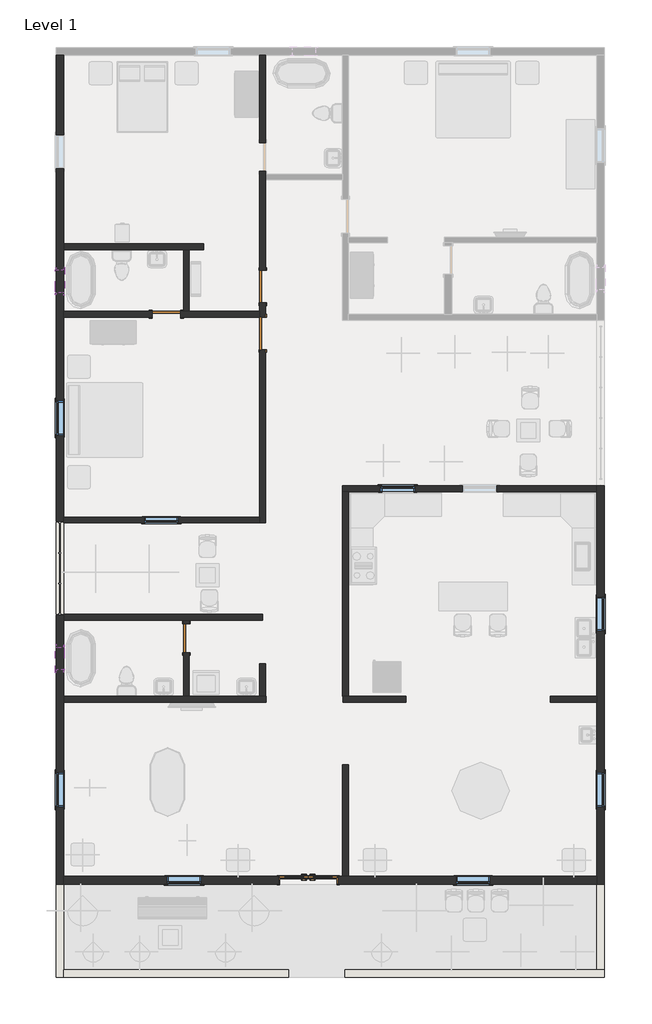
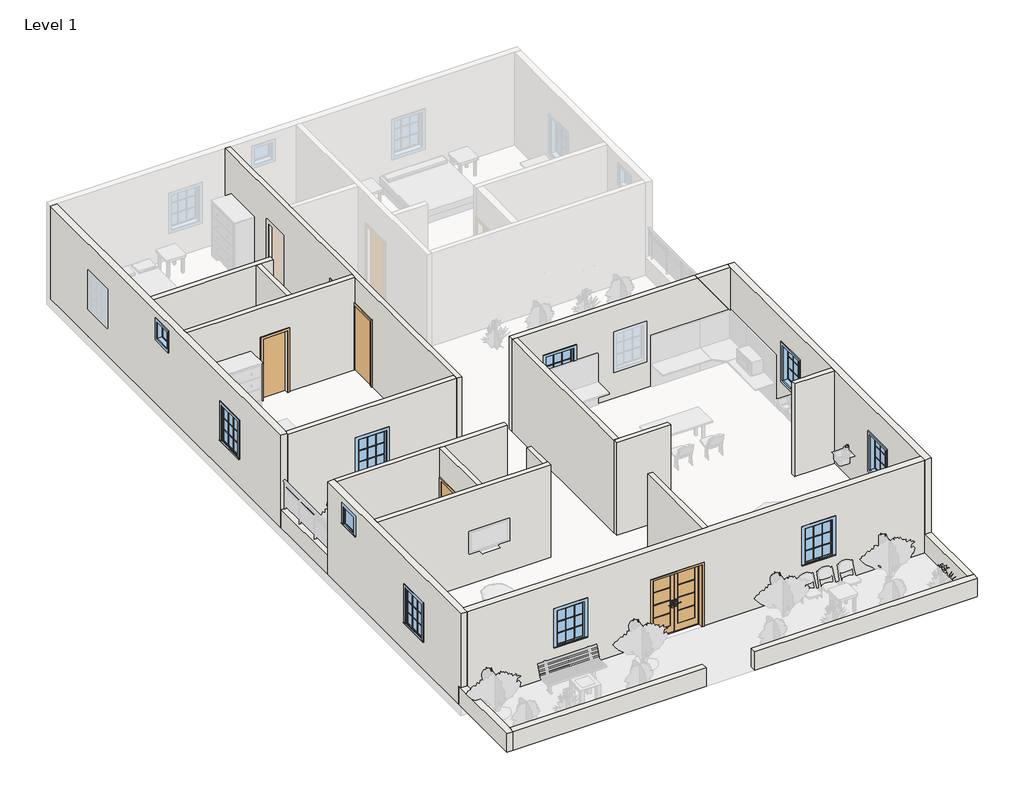
# One storey, part 1 of 3: 23 walls, 10 windows, 5 doors.
"""IFC4 building model written with IfcOpenShell, lengths in millimetres."""

from ifc_helpers import new_model, si_unit, frame, origin, origin_with_axes, place, context, project, spatial, polyline, outline, extrude, faceted_brep, transform, mapped, element, save
from components import door_b03bd389, door_059fdd7e, door_99d96fc5, door_b6e9fca3, window_29c06734, window_5c190c7e, window_e41d21a6

model = new_model("IFC4")

# Units and contexts
model_context = context("Model", 3, world=origin())
ifc_project = project(units=[si_unit("LENGTHUNIT", "METRE", prefix="MILLI")], contexts=[model_context])

# Site, building, storey
site = spatial("IfcSite", under=ifc_project)
building = spatial("IfcBuilding", under=site)
storey = spatial("IfcBuildingStorey", under=building, Name="Level 1", Elevation=0.0)

# Doors
placement = place(None, origin())
door_shape = door_b03bd389(model_context)
element("IfcDoor", 1, ObjectType="Door-Exterior-Double-Full Glass-Wood_Clad : 60\" x 80\"", at=placement, inside=storey, context=model_context, shape_type="MappedRepresentation", body=[
    mapped(door_shape, transform((-8336.7446525, -9537.1247829, 0.0), x_axis=(1.0, 0.0, 0.0), y_axis=(0.0, 1.0, 0.0), z_axis=(0.0, 0.0, 1.0))),
])
door_2_shape = door_059fdd7e(model_context)
element("IfcDoor", 2, ObjectType="Single-Flush : 30\" x 80\"", at=placement, inside=storey, context=model_context, shape_type="MappedRepresentation", body=[
    mapped(door_2_shape, transform((-12121.3446525, 5547.3002171, 0.0), x_axis=(1.0, 0.0, 0.0), y_axis=(0.0, 1.0, 0.0), z_axis=(0.0, 0.0, 1.0))),
])
element("IfcDoor", 3, ObjectType="Single-Flush : 30\" x 80\"", at=placement, inside=storey, context=model_context, shape_type="MappedRepresentation", body=[
    mapped(door_2_shape, transform((-11587.9446525, -3088.6997829, 0.0), x_axis=(0.0, 1.0, 0.0), y_axis=(-1.0, 0.0, 0.0), z_axis=(0.0, 0.0, 1.0))),
])
door_3_shape = door_99d96fc5(model_context)
element("IfcDoor", 4, ObjectType="Single-Flush : 34\" x 84\"", at=placement, inside=storey, context=model_context, shape_type="MappedRepresentation", body=[
    mapped(door_3_shape, transform((-9555.9446525, 6283.9002171, 0.0), x_axis=(0.0, -1.0, 0.0), y_axis=(1.0, 0.0, 0.0), z_axis=(0.0, 0.0, 1.0))),
])
door_4_shape = door_b6e9fca3(model_context)
element("IfcDoor", 5, ObjectType="Single-Flush : 34\" x 84\"", at=placement, inside=storey, context=model_context, shape_type="MappedRepresentation", body=[
    mapped(door_4_shape, transform((-9555.9446525, 5039.3002171, 0.0), x_axis=(0.0, 1.0, 0.0), y_axis=(-1.0, 0.0, 0.0), z_axis=(0.0, 0.0, 1.0))),
])

# Walls
element("IfcWall", 6, ObjectType="Generic - 2'", at=placement, inside=storey, context=model_context, shape_type="Brep", body=[
    faceted_brep([(-14864.5446525, -12131.0997829, 0.0), (-14864.5446525, -11927.8997829, 0.0), (-14864.5446525, -9641.8997829, 0.0), (-14864.5446525, -9540.2997829, 0.0), (-14864.5446525, -9540.2997829, 609.6), (-14864.5446525, -11927.8997829, 609.6), (-14864.5446525, -12131.0997829, 609.6), (-15067.7446525, -12131.0997829, 0.0), (-15067.7446525, -12131.0997829, 609.6), (-15067.7446525, -9540.2997829, 609.6), (-15067.7446525, -9540.2997829, 0.0)], [[[0, 1, 2, 3, 4, 5, 6]], [[7, 8, 9, 10]], [[3, 2, 1, 0, 7, 10]], [[4, 3, 10, 9]], [[6, 5, 4, 9, 8]], [[0, 6, 8, 7]]]),
])
element("IfcWall", 7, ObjectType="Generic - 2'", at=placement, inside=storey, context=model_context, shape_type="SweptSolid", body=[
    extrude(outline(polyline([(-14864.5446525, 10.1002171), (-14864.5446525, -2453.6997829), (-15067.7446525, -2453.6997829), (-15067.7446525, 10.1002171), (-14864.5446525, 10.1002171)])), origin_with_axes(), (0.0, 0.0, 1.0), 609.6),
])
element("IfcWall", 8, ObjectType="Generic - 2'", at=placement, inside=storey, context=model_context, shape_type="SweptSolid", body=[
    extrude(outline(polyline([(-8870.1446525, -12131.0997829), (-14864.5446525, -12131.0997829), (-14864.5446525, -11927.8997829), (-8870.1446525, -11927.8997829), (-8870.1446525, -12131.0997829)])), origin_with_axes(), (0.0, 0.0, 1.0), 609.6),
])
element("IfcWall", 9, ObjectType="Generic - 2'", at=placement, inside=storey, context=model_context, shape_type="Brep", body=[
    faceted_brep([(-7358.8446525, -12131.0997829, 0.0), (-437.3446525, -12131.0997829, 0.0), (-437.3446525, -12131.0997829, 609.6), (-7358.8446525, -12131.0997829, 609.6), (-7358.8446525, -11927.8997829, 0.0), (-7358.8446525, -11927.8997829, 609.6), (-640.5446525, -11927.8997829, 609.6), (-437.3446525, -11927.8997829, 609.6), (-437.3446525, -11927.8997829, 0.0), (-640.5446525, -11927.8997829, 0.0)], [[[0, 1, 2, 3]], [[4, 5, 6, 7, 8, 9]], [[1, 0, 4, 9, 8]], [[3, 2, 7, 6, 5]], [[0, 3, 5, 4]], [[2, 1, 8, 7]]]),
])
element("IfcWall", 10, ObjectType="Generic - 2'", at=placement, inside=storey, context=model_context, shape_type="Brep", body=[
    faceted_brep([(-640.5446525, -9540.2997829, 0.0), (-640.5446525, -9641.8997829, 0.0), (-640.5446525, -11927.8997829, 0.0), (-640.5446525, -11927.8997829, 609.6), (-640.5446525, -9540.2997829, 609.6), (-437.3446525, -9540.2997829, 0.0), (-437.3446525, -9540.2997829, 609.6), (-437.3446525, -11927.8997829, 609.6), (-437.3446525, -11927.8997829, 0.0)], [[[0, 1, 2, 3, 4]], [[5, 6, 7, 8]], [[2, 1, 0, 5, 8]], [[4, 3, 7, 6]], [[0, 4, 6, 5]], [[3, 2, 8, 7]]]),
])
element("IfcWall", 11, ObjectType="Generic - 8\"", at=placement, inside=storey, context=model_context, shape_type="Brep", body=[
    faceted_brep([(-14864.5446525, -9641.8997829, 3048.0), (-14864.5446525, -9641.8997829, 609.6), (-14864.5446525, -9641.8997829, 0.0), (-9124.1446525, -9641.8997829, 0.0), (-9124.1446525, -9641.8997829, 2057.4), (-7549.3446525, -9641.8997829, 2057.4), (-7549.3446525, -9641.8997829, 0.0), (-640.5446525, -9641.8997829, 0.0), (-640.5446525, -9641.8997829, 609.6), (-640.5446525, -9641.8997829, 3048.0), (-12108.6446525, -9641.8997829, 2133.6), (-11194.2446525, -9641.8997829, 2133.6), (-11194.2446525, -9641.8997829, 914.4), (-12108.6446525, -9641.8997829, 914.4), (-4399.7446525, -9641.8997829, 2133.6), (-3485.3446525, -9641.8997829, 2133.6), (-3485.3446525, -9641.8997829, 914.4), (-4399.7446525, -9641.8997829, 914.4), (-14864.5446525, -9438.6997829, 0.0), (-14864.5446525, -9438.6997829, 3048.0), (-7422.3446525, -9438.6997829, 3048.0), (-7269.9446525, -9438.6997829, 3048.0), (-640.5446525, -9438.6997829, 3048.0), (-640.5446525, -9438.6997829, 0.0), (-7269.9446525, -9438.6997829, 0.0), (-7422.3446525, -9438.6997829, 0.0), (-7549.3446525, -9438.6997829, 0.0), (-7549.3446525, -9438.6997829, 2057.4), (-9124.1446525, -9438.6997829, 2057.4), (-9124.1446525, -9438.6997829, 0.0), (-12108.6446525, -9438.6997829, 2133.6), (-12108.6446525, -9438.6997829, 914.4), (-11194.2446525, -9438.6997829, 914.4), (-11194.2446525, -9438.6997829, 2133.6), (-4399.7446525, -9438.6997829, 2133.6), (-4399.7446525, -9438.6997829, 914.4), (-3485.3446525, -9438.6997829, 914.4), (-3485.3446525, -9438.6997829, 2133.6), (-640.5446525, -9540.2997829, 0.0), (-14864.5446525, -9540.2997829, 0.0)], [[[0, 1, 2, 3, 4, 5, 6, 7, 8, 9], [10, 11, 12, 13], [14, 15, 16, 17]], [[18, 19, 20, 21, 22, 23, 24, 25, 26, 27, 28, 29], [30, 31, 32, 33], [34, 35, 36, 37]], [[23, 38, 7, 6, 26, 25, 24]], [[2, 39, 18, 29, 3]], [[5, 27, 26, 6]], [[27, 5, 4, 28]], [[28, 4, 3, 29]], [[31, 30, 10, 13]], [[32, 31, 13, 12]], [[33, 32, 12, 11]], [[30, 33, 11, 10]], [[35, 34, 14, 17]], [[36, 35, 17, 16]], [[37, 36, 16, 15]], [[34, 37, 15, 14]], [[18, 39, 2, 1, 0, 19]], [[7, 38, 23, 22, 9, 8]], [[0, 9, 22, 21, 20, 19]]]),
])
element("IfcWall", 12, ObjectType="Generic - 8\"", at=placement, inside=storey, context=model_context, shape_type="Brep", body=[
    faceted_brep([(-14864.5446525, 35.5002171, 0.0), (-14864.5446525, 137.1002171, 0.0), (-14864.5446525, 5471.1002171, 0.0), (-14864.5446525, 5623.5002171, 0.0), (-14864.5446525, 7274.5002171, 0.0), (-14864.5446525, 7426.9002171, 0.0), (-14864.5446525, 12456.1002171, 0.0), (-14864.5446525, 12456.1002171, 3048.0), (-14864.5446525, 7426.9002171, 3048.0), (-14864.5446525, 7274.5002171, 3048.0), (-14864.5446525, 5623.5002171, 3048.0), (-14864.5446525, 5471.1002171, 3048.0), (-14864.5446525, 137.1002171, 3048.0), (-14864.5446525, 35.5002171, 3048.0), (-14864.5446525, 10335.2002171, 2133.6), (-14864.5446525, 10335.2002171, 914.4), (-14864.5446525, 9420.8002171, 914.4), (-14864.5446525, 9420.8002171, 2133.6), (-14864.5446525, 3235.9002171, 2133.6), (-14864.5446525, 3235.9002171, 914.4), (-14864.5446525, 2321.5002171, 914.4), (-14864.5446525, 2321.5002171, 2133.6), (-14864.5446525, 6118.8002171, 2768.6), (-14864.5446525, 6728.4002171, 2768.6), (-14864.5446525, 6728.4002171, 2159.0), (-14864.5446525, 6118.8002171, 2159.0), (-15067.7446525, 35.5002171, 0.0), (-15067.7446525, 35.5002171, 3048.0), (-15067.7446525, 12456.1002171, 3048.0), (-15067.7446525, 12456.1002171, 0.0), (-15067.7446525, 10335.2002171, 2133.6), (-15067.7446525, 9420.8002171, 2133.6), (-15067.7446525, 9420.8002171, 914.4), (-15067.7446525, 10335.2002171, 914.4), (-15067.7446525, 3235.9002171, 2133.6), (-15067.7446525, 2321.5002171, 2133.6), (-15067.7446525, 2321.5002171, 914.4), (-15067.7446525, 3235.9002171, 914.4), (-15067.7446525, 6118.8002171, 2768.6), (-15067.7446525, 6118.8002171, 2159.0), (-15067.7446525, 6728.4002171, 2159.0), (-15067.7446525, 6728.4002171, 2768.6)], [[[0, 1, 2, 3, 4, 5, 6, 7, 8, 9, 10, 11, 12, 13], [14, 15, 16, 17], [18, 19, 20, 21], [22, 23, 24, 25]], [[26, 27, 28, 29], [30, 31, 32, 33], [34, 35, 36, 37], [38, 39, 40, 41]], [[6, 5, 4, 3, 2, 1, 0, 26, 29]], [[0, 13, 27, 26]], [[7, 6, 29, 28]], [[15, 14, 30, 33]], [[16, 15, 33, 32]], [[17, 16, 32, 31]], [[14, 17, 31, 30]], [[19, 18, 34, 37]], [[20, 19, 37, 36]], [[21, 20, 36, 35]], [[18, 21, 35, 34]], [[39, 38, 22, 25]], [[40, 39, 25, 24]], [[41, 40, 24, 23]], [[38, 41, 23, 22]], [[13, 12, 11, 10, 9, 8, 7, 28, 27]]]),
])
element("IfcWall", 13, ObjectType="Generic - 8\"", at=placement, inside=storey, context=model_context, shape_type="Brep", body=[
    faceted_brep([(-640.5446525, 899.1002171, 0.0), (-640.5446525, 822.9002171, 0.0), (-640.5446525, -4638.0997829, 0.0), (-640.5446525, -4790.4997829, 0.0), (-640.5446525, -9438.6997829, 0.0), (-640.5446525, -9540.2997829, 0.0), (-640.5446525, -9540.2997829, 609.6), (-640.5446525, -9641.8997829, 609.6), (-640.5446525, -9641.8997829, 3048.0), (-640.5446525, -9438.6997829, 3048.0), (-640.5446525, -4790.4997829, 3048.0), (-640.5446525, -4638.0997829, 3048.0), (-640.5446525, 822.9002171, 3048.0), (-640.5446525, 975.3002171, 3048.0), (-640.5446525, 975.3002171, 609.6), (-640.5446525, 899.1002171, 609.6), (-640.5446525, -7584.4997829, 2133.6), (-640.5446525, -7584.4997829, 914.4), (-640.5446525, -6670.0997829, 914.4), (-640.5446525, -6670.0997829, 2133.6), (-640.5446525, -2898.1997829, 2228.85), (-640.5446525, -2898.1997829, 1009.65), (-640.5446525, -1983.7997829, 1009.65), (-640.5446525, -1983.7997829, 2228.85), (-437.3446525, 899.1002171, 0.0), (-437.3446525, 899.1002171, 609.6), (-437.3446525, 975.3002171, 609.6), (-437.3446525, 975.3002171, 3048.0), (-437.3446525, -9641.8997829, 3048.0), (-437.3446525, -9641.8997829, 609.6), (-437.3446525, -9540.2997829, 609.6), (-437.3446525, -9540.2997829, 0.0), (-437.3446525, -7584.4997829, 2133.6), (-437.3446525, -6670.0997829, 2133.6), (-437.3446525, -6670.0997829, 914.4), (-437.3446525, -7584.4997829, 914.4), (-437.3446525, -2898.1997829, 2228.85), (-437.3446525, -1983.7997829, 2228.85), (-437.3446525, -1983.7997829, 1009.65), (-437.3446525, -2898.1997829, 1009.65)], [[[0, 1, 2, 3, 4, 5, 6, 7, 8, 9, 10, 11, 12, 13, 14, 15], [16, 17, 18, 19], [20, 21, 22, 23]], [[24, 25, 26, 27, 28, 29, 30, 31], [32, 33, 34, 35], [36, 37, 38, 39]], [[5, 4, 3, 2, 1, 0, 24, 31]], [[16, 19, 33, 32]], [[19, 18, 34, 33]], [[18, 17, 35, 34]], [[17, 16, 32, 35]], [[20, 23, 37, 36]], [[23, 22, 38, 37]], [[22, 21, 39, 38]], [[21, 20, 36, 39]], [[0, 15, 25, 24]], [[14, 26, 25, 15]], [[14, 13, 27, 26]], [[6, 5, 31, 30]], [[29, 7, 6, 30]], [[8, 7, 29, 28]], [[13, 12, 11, 10, 9, 8, 28, 27]]]),
])
element("IfcWall", 14, ObjectType="Generic - 8\"", at=placement, inside=storey, context=model_context, shape_type="Brep", body=[
    faceted_brep([(-14864.5446525, -9540.2997829, 0.0), (-14864.5446525, -9438.6997829, 0.0), (-14864.5446525, -4790.4997829, 0.0), (-14864.5446525, -4638.0997829, 0.0), (-14864.5446525, -2606.0997829, 0.0), (-14864.5446525, -2479.0997829, 0.0), (-14864.5446525, -2479.0997829, 3048.0), (-14864.5446525, -2606.0997829, 3048.0), (-14864.5446525, -4638.0997829, 3048.0), (-14864.5446525, -4790.4997829, 3048.0), (-14864.5446525, -9438.6997829, 3048.0), (-14864.5446525, -9641.8997829, 3048.0), (-14864.5446525, -9641.8997829, 609.6), (-14864.5446525, -9540.2997829, 609.6), (-14864.5446525, -6670.0997829, 2133.6), (-14864.5446525, -6670.0997829, 914.4), (-14864.5446525, -7584.4997829, 914.4), (-14864.5446525, -7584.4997829, 2133.6), (-14864.5446525, -3323.6497829, 2768.6), (-14864.5446525, -3323.6497829, 2159.0), (-14864.5446525, -3933.2497829, 2159.0), (-14864.5446525, -3933.2497829, 2768.6), (-15067.7446525, -9540.2997829, 0.0), (-15067.7446525, -9540.2997829, 609.6), (-15067.7446525, -9641.8997829, 609.6), (-15067.7446525, -9641.8997829, 3048.0), (-15067.7446525, -2479.0997829, 3048.0), (-15067.7446525, -2479.0997829, 0.0), (-15067.7446525, -6670.0997829, 2133.6), (-15067.7446525, -7584.4997829, 2133.6), (-15067.7446525, -7584.4997829, 914.4), (-15067.7446525, -6670.0997829, 914.4), (-15067.7446525, -3323.6497829, 2768.6), (-15067.7446525, -3933.2497829, 2768.6), (-15067.7446525, -3933.2497829, 2159.0), (-15067.7446525, -3323.6497829, 2159.0)], [[[0, 1, 2, 3, 4, 5, 6, 7, 8, 9, 10, 11, 12, 13], [14, 15, 16, 17], [18, 19, 20, 21]], [[22, 23, 24, 25, 26, 27], [28, 29, 30, 31], [32, 33, 34, 35]], [[5, 4, 3, 2, 1, 0, 22, 27]], [[6, 5, 27, 26]], [[14, 17, 29, 28]], [[17, 16, 30, 29]], [[16, 15, 31, 30]], [[15, 14, 28, 31]], [[18, 21, 33, 32]], [[21, 20, 34, 33]], [[20, 19, 35, 34]], [[19, 18, 32, 35]], [[0, 13, 23, 22]], [[12, 24, 23, 13]], [[12, 11, 25, 24]], [[11, 10, 9, 8, 7, 6, 26, 25]]]),
])
element("IfcWall", 15, ObjectType="INNER 6\"", at=placement, inside=storey, context=model_context, shape_type="SweptSolid", body=[
    extrude(outline(polyline([(-1885.1446525, -4638.0997829), (-640.5446525, -4638.0997829), (-640.5446525, -4790.4997829), (-1885.1446525, -4790.4997829), (-1885.1446525, -4638.0997829)])), origin_with_axes(), (0.0, 0.0, 1.0), 3048.0),
])
element("IfcWall", 16, ObjectType="INNER 6\"", at=placement, inside=storey, context=model_context, shape_type="Brep", body=[
    faceted_brep([(-9632.1446525, 5852.1002171, 0.0), (-9632.1446525, 5623.5002171, 0.0), (-9632.1446525, 5471.1002171, 0.0), (-9632.1446525, 5471.1002171, 2133.6), (-9632.1446525, 4607.5002171, 2133.6), (-9632.1446525, 4607.5002171, 0.0), (-9632.1446525, 137.1002171, 0.0), (-9632.1446525, -15.2997829, 0.0), (-9632.1446525, -15.2997829, 3048.0), (-9632.1446525, 137.1002171, 3048.0), (-9632.1446525, 5471.1002171, 3048.0), (-9632.1446525, 5623.5002171, 3048.0), (-9632.1446525, 12456.1002171, 3048.0), (-9632.1446525, 12456.1002171, 0.0), (-9632.1446525, 10119.3002171, 0.0), (-9632.1446525, 10119.3002171, 2032.0), (-9632.1446525, 9357.3002171, 2032.0), (-9632.1446525, 9357.3002171, 0.0), (-9632.1446525, 6715.7002171, 0.0), (-9632.1446525, 6715.7002171, 2133.6), (-9632.1446525, 5852.1002171, 2133.6), (-9479.7446525, 5471.1002171, 2133.6), (-9479.7446525, 5471.1002171, 0.0), (-9479.7446525, 5852.1002171, 0.0), (-9479.7446525, 5852.1002171, 2133.6), (-9479.7446525, 6715.7002171, 2133.6), (-9479.7446525, 6715.7002171, 0.0), (-9479.7446525, 9128.7002171, 0.0), (-9479.7446525, 9281.1002171, 0.0), (-9479.7446525, 9357.3002171, 0.0), (-9479.7446525, 9357.3002171, 2032.0), (-9479.7446525, 10119.3002171, 2032.0), (-9479.7446525, 10119.3002171, 0.0), (-9479.7446525, 12456.1002171, 0.0), (-9479.7446525, 12456.1002171, 3048.0), (-9479.7446525, 9281.1002171, 3048.0), (-9479.7446525, 9128.7002171, 3048.0), (-9479.7446525, -15.2997829, 3048.0), (-9479.7446525, -15.2997829, 0.0), (-9479.7446525, 4607.5002171, 0.0), (-9479.7446525, 4607.5002171, 2133.6)], [[[0, 1, 2, 3, 4, 5, 6, 7, 8, 9, 10, 11, 12, 13, 14, 15, 16, 17, 18, 19, 20]], [[21, 22, 23, 24, 25, 26, 27, 28, 29, 30, 31, 32, 33, 34, 35, 36, 37, 38, 39, 40]], [[14, 13, 33, 32]], [[18, 17, 29, 28, 27, 26]], [[39, 38, 7, 6, 5]], [[23, 22, 2, 1, 0]], [[13, 12, 34, 33]], [[8, 7, 38, 37]], [[30, 29, 17, 16]], [[31, 30, 16, 15]], [[32, 31, 15, 14]], [[24, 23, 0, 20]], [[25, 24, 20, 19]], [[26, 25, 19, 18]], [[3, 2, 22, 21]], [[4, 3, 21, 40]], [[5, 4, 40, 39]], [[12, 11, 10, 9, 8, 37, 36, 35, 34]]]),
])
element("IfcWall", 17, ObjectType="INNER 6\"", at=placement, inside=storey, context=model_context, shape_type="Brep", body=[
    faceted_brep([(-9632.1446525, 5623.5002171, 0.0), (-11511.7446525, 5623.5002171, 0.0), (-11664.1446525, 5623.5002171, 0.0), (-11740.3446525, 5623.5002171, 0.0), (-11740.3446525, 5623.5002171, 2032.0), (-12502.3446525, 5623.5002171, 2032.0), (-12502.3446525, 5623.5002171, 0.0), (-14864.5446525, 5623.5002171, 0.0), (-14864.5446525, 5623.5002171, 3048.0), (-11664.1446525, 5623.5002171, 3048.0), (-11511.7446525, 5623.5002171, 3048.0), (-9632.1446525, 5623.5002171, 3048.0), (-11740.3446525, 5471.1002171, 2032.0), (-11740.3446525, 5471.1002171, 0.0), (-9632.1446525, 5471.1002171, 0.0), (-9632.1446525, 5471.1002171, 2133.6), (-9632.1446525, 5471.1002171, 3048.0), (-14864.5446525, 5471.1002171, 3048.0), (-14864.5446525, 5471.1002171, 0.0), (-12502.3446525, 5471.1002171, 0.0), (-12502.3446525, 5471.1002171, 2032.0)], [[[0, 1, 2, 3, 4, 5, 6, 7, 8, 9, 10, 11]], [[12, 13, 14, 15, 16, 17, 18, 19, 20]], [[19, 18, 7, 6]], [[14, 13, 3, 2, 1, 0]], [[0, 11, 16, 15, 14]], [[8, 7, 18, 17]], [[4, 3, 13, 12]], [[5, 4, 12, 20]], [[6, 5, 20, 19]], [[11, 10, 9, 8, 17, 16]]]),
])
element("IfcWall", 18, ObjectType="INNER 6\"", at=placement, inside=storey, context=model_context, shape_type="Brep", body=[
    faceted_brep([(-14864.5446525, 7274.5002171, 0.0), (-11664.1446525, 7274.5002171, 0.0), (-11511.7446525, 7274.5002171, 0.0), (-11130.7446525, 7274.5002171, 0.0), (-11130.7446525, 7274.5002171, 3048.0), (-11511.7446525, 7274.5002171, 3048.0), (-11664.1446525, 7274.5002171, 3048.0), (-14864.5446525, 7274.5002171, 3048.0), (-14864.5446525, 7426.9002171, 0.0), (-14864.5446525, 7426.9002171, 3048.0), (-11130.7446525, 7426.9002171, 3048.0), (-11130.7446525, 7426.9002171, 0.0)], [[[0, 1, 2, 3, 4, 5, 6, 7]], [[8, 9, 10, 11]], [[3, 2, 1, 0, 8, 11]], [[4, 3, 11, 10]], [[0, 7, 9, 8]], [[7, 6, 5, 4, 10, 9]]]),
])
element("IfcWall", 19, ObjectType="INNER 6\"", at=placement, inside=storey, context=model_context, shape_type="SweptSolid", body=[
    extrude(outline(polyline([(-11664.1446525, 5623.5002171), (-11664.1446525, 7274.5002171), (-11511.7446525, 7274.5002171), (-11511.7446525, 5623.5002171), (-11664.1446525, 5623.5002171)])), origin_with_axes(), (0.0, 0.0, 1.0), 3048.0),
])
element("IfcWall", 20, ObjectType="INNER 6\"", at=placement, inside=storey, context=model_context, shape_type="Brep", body=[
    faceted_brep([(-9632.1446525, 137.1002171, 0.0), (-14864.5446525, 137.1002171, 0.0), (-14864.5446525, 137.1002171, 3048.0), (-9632.1446525, 137.1002171, 3048.0), (-12718.2446525, 137.1002171, 2133.6), (-12718.2446525, 137.1002171, 914.4), (-11803.8446525, 137.1002171, 914.4), (-11803.8446525, 137.1002171, 2133.6), (-9632.1446525, -15.2997829, 0.0), (-9632.1446525, -15.2997829, 3048.0), (-14864.5446525, -15.2997829, 3048.0), (-14864.5446525, -15.2997829, 0.0), (-12718.2446525, -15.2997829, 2133.6), (-11803.8446525, -15.2997829, 2133.6), (-11803.8446525, -15.2997829, 914.4), (-12718.2446525, -15.2997829, 914.4), (-14864.5446525, 35.5002171, 0.0), (-14864.5446525, 35.5002171, 3048.0)], [[[0, 1, 2, 3], [4, 5, 6, 7]], [[8, 9, 10, 11], [12, 13, 14, 15]], [[1, 0, 8, 11, 16]], [[0, 3, 9, 8]], [[2, 1, 16, 11, 10, 17]], [[5, 4, 12, 15]], [[6, 5, 15, 14]], [[7, 6, 14, 13]], [[4, 7, 13, 12]], [[3, 2, 17, 10, 9]]]),
])
element("IfcWall", 21, ObjectType="INNER 6\"", at=placement, inside=storey, context=model_context, shape_type="Brep", body=[
    faceted_brep([(-9555.9446525, -2453.6997829, 0.0), (-14864.5446525, -2453.6997829, 0.0), (-14864.5446525, -2453.6997829, 3048.0), (-9555.9446525, -2453.6997829, 3048.0), (-9555.9446525, -2606.0997829, 0.0), (-9555.9446525, -2606.0997829, 3048.0), (-11511.7446525, -2606.0997829, 3048.0), (-11664.1446525, -2606.0997829, 3048.0), (-14864.5446525, -2606.0997829, 3048.0), (-14864.5446525, -2606.0997829, 0.0), (-11664.1446525, -2606.0997829, 0.0), (-11511.7446525, -2606.0997829, 0.0), (-14864.5446525, -2479.0997829, 0.0), (-14864.5446525, -2479.0997829, 3048.0)], [[[0, 1, 2, 3]], [[4, 5, 6, 7, 8, 9, 10, 11]], [[1, 0, 4, 11, 10, 9, 12]], [[0, 3, 5, 4]], [[2, 1, 12, 9, 8, 13]], [[3, 2, 13, 8, 7, 6, 5]]]),
])
element("IfcWall", 22, ObjectType="INNER 6\"", at=placement, inside=storey, context=model_context, shape_type="SweptSolid", body=[
    extrude(outline(polyline([(-2606.0997829, 0.0), (-2707.6997829, 0.0), (-2707.6997829, 2032.0), (-3469.6997829, 2032.0), (-3469.6997829, 0.0), (-4638.0997829, 0.0), (-4638.0997829, 3048.0), (-2606.0997829, 3048.0), (-2606.0997829, 0.0)])), frame((-11664.1446525, 0.0, 0.0), z_axis=(1.0, 0.0, 0.0), x_axis=(0.0, 1.0, 0.0)), (0.0, 0.0, 1.0), 152.4),
])
element("IfcWall", 23, ObjectType="INNER 6\"", at=placement, inside=storey, context=model_context, shape_type="Brep", body=[
    faceted_brep([(-7422.3446525, 822.9002171, 0.0), (-7269.9446525, 822.9002171, 0.0), (-640.5446525, 822.9002171, 0.0), (-640.5446525, 822.9002171, 3048.0), (-7269.9446525, 822.9002171, 3048.0), (-7422.3446525, 822.9002171, 3048.0), (-3307.5446525, 822.9002171, 2133.6), (-3307.5446525, 822.9002171, 914.4), (-4221.9446525, 822.9002171, 914.4), (-4221.9446525, 822.9002171, 2133.6), (-5491.9446525, 822.9002171, 2133.6), (-5491.9446525, 822.9002171, 914.4), (-6406.3446525, 822.9002171, 914.4), (-6406.3446525, 822.9002171, 2133.6), (-7422.3446525, 975.3002171, 0.0), (-7422.3446525, 975.3002171, 3048.0), (-640.5446525, 975.3002171, 3048.0), (-640.5446525, 975.3002171, 609.6), (-640.5446525, 975.3002171, 0.0), (-3307.5446525, 975.3002171, 2133.6), (-4221.9446525, 975.3002171, 2133.6), (-4221.9446525, 975.3002171, 914.4), (-3307.5446525, 975.3002171, 914.4), (-5491.9446525, 975.3002171, 2133.6), (-6406.3446525, 975.3002171, 2133.6), (-6406.3446525, 975.3002171, 914.4), (-5491.9446525, 975.3002171, 914.4), (-640.5446525, 899.1002171, 0.0)], [[[0, 1, 2, 3, 4, 5], [6, 7, 8, 9], [10, 11, 12, 13]], [[14, 15, 16, 17, 18], [19, 20, 21, 22], [23, 24, 25, 26]], [[2, 1, 0, 14, 18, 27]], [[0, 5, 15, 14]], [[7, 6, 19, 22]], [[8, 7, 22, 21]], [[9, 8, 21, 20]], [[6, 9, 20, 19]], [[11, 10, 23, 26]], [[12, 11, 26, 25]], [[13, 12, 25, 24]], [[10, 13, 24, 23]], [[2, 27, 18, 17, 16, 3]], [[5, 4, 3, 16, 15]]]),
])
element("IfcWall", 24, ObjectType="INNER 6\"", at=placement, inside=storey, context=model_context, shape_type="Brep", body=[
    faceted_brep([(-7422.3446525, 822.9002171, 0.0), (-7422.3446525, -4638.0997829, 0.0), (-7422.3446525, -4638.0997829, 3048.0), (-7422.3446525, 822.9002171, 3048.0), (-7269.9446525, 822.9002171, 0.0), (-7269.9446525, 822.9002171, 3048.0), (-7269.9446525, -4638.0997829, 3048.0), (-7269.9446525, -4638.0997829, 0.0), (-7409.6446525, -4638.0997829, 0.0), (-7409.6446525, -4638.0997829, 3048.0)], [[[0, 1, 2, 3]], [[4, 5, 6, 7]], [[1, 0, 4, 7, 8]], [[0, 3, 5, 4]], [[2, 1, 8, 7, 6, 9]], [[3, 2, 9, 6, 5]]]),
])
element("IfcWall", 25, ObjectType="INNER 6\"", at=placement, inside=storey, context=model_context, shape_type="SweptSolid", body=[
    extrude(outline(polyline([(-7422.3446525, -9438.6997829), (-7422.3446525, -6466.8997829), (-7269.9446525, -6466.8997829), (-7269.9446525, -9438.6997829), (-7422.3446525, -9438.6997829)])), origin_with_axes(), (0.0, 0.0, 1.0), 3048.0),
])
element("IfcWall", 26, ObjectType="INNER 6\"", at=placement, inside=storey, context=model_context, shape_type="SweptSolid", body=[
    extrude(outline(polyline([(-9632.1446525, -4638.0997829), (-9632.1446525, -3774.4997829), (-9479.7446525, -3774.4997829), (-9479.7446525, -4638.0997829), (-9632.1446525, -4638.0997829)])), origin_with_axes(), (0.0, 0.0, 1.0), 3048.0),
])
element("IfcWall", 27, ObjectType="INNER 6\"", at=placement, inside=storey, context=model_context, shape_type="Brep", body=[
    faceted_brep([(-9467.0446525, -4638.0997829, 0.0), (-9479.7446525, -4638.0997829, 0.0), (-9632.1446525, -4638.0997829, 0.0), (-11511.7446525, -4638.0997829, 0.0), (-11664.1446525, -4638.0997829, 0.0), (-14864.5446525, -4638.0997829, 0.0), (-14864.5446525, -4638.0997829, 3048.0), (-11664.1446525, -4638.0997829, 3048.0), (-11511.7446525, -4638.0997829, 3048.0), (-9632.1446525, -4638.0997829, 3048.0), (-9479.7446525, -4638.0997829, 3048.0), (-9467.0446525, -4638.0997829, 3048.0), (-9467.0446525, -4790.4997829, 0.0), (-9467.0446525, -4790.4997829, 3048.0), (-14864.5446525, -4790.4997829, 3048.0), (-14864.5446525, -4790.4997829, 0.0)], [[[0, 1, 2, 3, 4, 5, 6, 7, 8, 9, 10, 11]], [[12, 13, 14, 15]], [[5, 4, 3, 2, 1, 0, 12, 15]], [[0, 11, 13, 12]], [[6, 5, 15, 14]], [[11, 10, 9, 8, 7, 6, 14, 13]]]),
])
element("IfcWall", 28, ObjectType="INNER 6\"", at=placement, inside=storey, context=model_context, shape_type="Brep", body=[
    faceted_brep([(-5733.2446525, -4638.0997829, 0.0), (-7269.9446525, -4638.0997829, 0.0), (-7409.6446525, -4638.0997829, 0.0), (-7409.6446525, -4638.0997829, 3048.0), (-7269.9446525, -4638.0997829, 3048.0), (-5733.2446525, -4638.0997829, 3048.0), (-5733.2446525, -4790.4997829, 0.0), (-5733.2446525, -4790.4997829, 3048.0), (-7409.6446525, -4790.4997829, 3048.0), (-7409.6446525, -4790.4997829, 0.0)], [[[0, 1, 2, 3, 4, 5]], [[6, 7, 8, 9]], [[2, 1, 0, 6, 9]], [[3, 2, 9, 8]], [[0, 5, 7, 6]], [[5, 4, 3, 8, 7]]]),
])

# Windows
window_shape = window_29c06734(model_context)
element("IfcWindow", 29, ObjectType="Casement 3x3 with Trim : 36\" x 48\"", at=placement, inside=storey, context=model_context, shape_type="MappedRepresentation", body=[
    mapped(window_shape, transform((-14966.1446525, 2778.7002171, 0.0), x_axis=(0.0, 1.0, 0.0), y_axis=(-1.0, 0.0, 0.0), z_axis=(0.0, 0.0, 1.0))),
])
element("IfcWindow", 30, ObjectType="Casement 3x3 with Trim : 36\" x 48\"", at=placement, inside=storey, context=model_context, shape_type="MappedRepresentation", body=[
    mapped(window_shape, transform((-14966.1446525, -7127.2997829, 0.0), x_axis=(0.0, 1.0, 0.0), y_axis=(-1.0, 0.0, 0.0), z_axis=(0.0, 0.0, 1.0))),
])
element("IfcWindow", 31, ObjectType="Casement 3x3 with Trim : 36\" x 48\"", at=placement, inside=storey, context=model_context, shape_type="MappedRepresentation", body=[
    mapped(window_shape, transform((-11651.4446525, -9540.2997829, 0.0), x_axis=(-1.0, 0.0, 0.0), y_axis=(0.0, -1.0, 0.0), z_axis=(0.0, 0.0, 1.0))),
])
element("IfcWindow", 32, ObjectType="Casement 3x3 with Trim : 36\" x 48\"", at=placement, inside=storey, context=model_context, shape_type="MappedRepresentation", body=[
    mapped(window_shape, transform((-3942.5446525, -9540.2997829, 0.0), x_axis=(-1.0, 0.0, 0.0), y_axis=(0.0, -1.0, 0.0), z_axis=(0.0, 0.0, 1.0))),
])
element("IfcWindow", 33, ObjectType="Casement 3x3 with Trim : 36\" x 48\"", at=placement, inside=storey, context=model_context, shape_type="MappedRepresentation", body=[
    mapped(window_shape, transform((-538.9446525, -7127.2997829, 0.0), x_axis=(0.0, -1.0, 0.0), y_axis=(1.0, 0.0, 0.0), z_axis=(0.0, 0.0, 1.0))),
])
element("IfcWindow", 34, ObjectType="Casement 3x3 with Trim : 36\" x 48\"", at=placement, inside=storey, context=model_context, shape_type="MappedRepresentation", body=[
    mapped(window_shape, transform((-538.9446525, -2440.9997829, 95.25), x_axis=(0.0, -1.0, 0.0), y_axis=(1.0, 0.0, 0.0), z_axis=(0.0, 0.0, 1.0))),
])
window_2_shape = window_5c190c7e(model_context)
element("IfcWindow", 35, ObjectType="Casement 3x3 with Trim : 36\" x 48\"", at=placement, inside=storey, context=model_context, shape_type="MappedRepresentation", body=[
    mapped(window_2_shape, transform((-12261.0446525, 60.9002171, 0.0), x_axis=(-1.0, 0.0, 0.0), y_axis=(0.0, -1.0, 0.0), z_axis=(0.0, 0.0, 1.0))),
])
element("IfcWindow", 36, ObjectType="Casement 3x3 with Trim : 36\" x 48\"", at=placement, inside=storey, context=model_context, shape_type="MappedRepresentation", body=[
    mapped(window_2_shape, transform((-5949.1446525, 899.1002171, 0.0), x_axis=(1.0, 0.0, 0.0), y_axis=(0.0, 1.0, 0.0), z_axis=(0.0, 0.0, 1.0))),
])
window_3_shape = window_e41d21a6(model_context)
element("IfcWindow", 37, ObjectType="Transom with Trim : 24\" x 24\"", at=placement, inside=storey, context=model_context, shape_type="MappedRepresentation", body=[
    mapped(window_3_shape, transform((-14966.1446525, 6385.5002171, 0.0), x_axis=(0.0, -1.0, 0.0), y_axis=(1.0, 0.0, 0.0), z_axis=(0.0, 0.0, 1.0))),
])
element("IfcWindow", 38, ObjectType="Transom with Trim : 24\" x 24\"", at=placement, inside=storey, context=model_context, shape_type="MappedRepresentation", body=[
    mapped(window_3_shape, transform((-14966.1446525, -3590.3497829, 0.0), x_axis=(0.0, 1.0, 0.0), y_axis=(-1.0, 0.0, 0.0), z_axis=(0.0, 0.0, 1.0))),
])

save(model, "model.ifc")

# Revit data of these elements
# Type "Door-Exterior-Double-Full Glass-Wood_Clad : 60\" x 80\""
#   Type Mark = "8"
#   Assembly Code = "B2030100"
#   Analytic Construction = "French door, wood frame with double glass"
#   Top Rail = 0' - 4 11/16"
#   Threshold Offset [instance default] = 0' - 0 1/2"
#   Thickness = 0' - 1 3/8"
#   Thermal Resistance (R) = 1.9158 (h·ft²·°F)/BTU
#   Swing Angle [instance default] = 90.00°
#   Stiles = 0' - 4 3/4"
#   Rough Width = 5' - 2"
#   Rough Height = 6' - 9"
#   Panel Width = 2' - 6"
#   Door Offset [instance default] = 0' - 0"
#   Height = 6' - 8"
#   Width = 5' - 0"
#   Heat Transfer Coefficient (U) = 0.5220 BTU/(h·ft²·°F)
#   Bottom Rail = 0' - 9 1/8"
#   Exterior Trim [instance default] = yes
#   Threshold [instance default] = yes
#   Show Grill [instance default] = yes
#   Function = 1
#   Trim Material = Cherry
#   Threshold Material = Cherry
#   Panel Material = Cherry
#   Glazing = Glass
#   Frame Material = Cherry
#   Door Handle Material = Aluminum
#   Visual Light Transmittance = 0
#   Solar Heat Gain Coefficient = 0
#   Wall Closure = (empty or 0)
#   Construction Type = (empty or 0)
# Type "Single-Flush : 30\" x 80\""
#   Type Mark = "5"
#   Construction Type Id = "MDOOR"
#   Assembly Code = "C1020"
#   Analytic Construction = "Metal"
#   Thickness = 0' - 2"
#   Heat Transfer Coefficient (U) = 0.651978 BTU/(h·ft²·°F)
#   Height = 6' - 8"
#   Trim Projection Ext = 0' - 1"
#   Trim Projection Int = 0' - 1"
#   Trim Width = 0' - 3"
#   Width = 2' - 6"
#   Define Thermal Properties by = 1
#   Door Material = Door - Panel
#   Frame Material = Door - Frame
#   Visual Light Transmittance = 0
#   Solar Heat Gain Coefficient = 0
#   Function = (empty or 0)
#   Wall Closure = (empty or 0)
# Type "Single-Flush : 34\" x 84\""
#   Type Mark = "2"
#   Construction Type Id = "MDOOR"
#   Assembly Code = "C1020"
#   Analytic Construction = "Metal"
#   Thickness = 0' - 2"
#   Heat Transfer Coefficient (U) = 0.651978 BTU/(h·ft²·°F)
#   Height = 7' - 0"
#   Trim Projection Ext = 0' - 1"
#   Trim Projection Int = 0' - 1"
#   Trim Width = 0' - 3"
#   Width = 2' - 10"
#   Define Thermal Properties by = 1
#   Door Material = Door - Panel
#   Frame Material = Door - Frame
#   Visual Light Transmittance = 0
#   Solar Heat Gain Coefficient = 0
#   Function = (empty or 0)
#   Wall Closure = (empty or 0)
# Type "Generic - 2'"
#   Assembly Code = "B2010"
#   Layers, outside or top first: 0' - 8" "Birch" (function 1)
# Type "Generic - 8\""
#   Assembly Code = "B2010"
#   Layers, outside or top first: 0' - 8" "Brick, Common" (function 1)
# Type "INNER 6\""
#   Assembly Code = "B2010"
#   Layers, outside or top first: 0' - 6" "Brick, Common" (function 1)
# Type "Casement 3x3 with Trim : 36\" x 48\""
#   Type Mark = "10"
#   Construction Type Id = "GSP4R"
#   Assembly Code = "B2020100"
#   Analytic Construction = "1/8 in Pilkington single glazing"
#   Visual Light Transmittance = 0.9
#   Solar Heat Gain Coefficient = 0.78
#   Heat Transfer Coefficient (U) = 0.6496 BTU/(h·ft²·°F)
#   Height = 4' - 0"
#   Default Sill Height = 3' - 0"
#   Trim Projection - Ext. = 0' - 0 1/2"
#   Trim Projection - Int. = 0' - 0 3/4"
#   Trim Width - Exterior = 0' - 3 1/2"
#   Trim Width - Interior = 0' - 3 1/2"
#   Width = 3' - 0"
#   Window Inset = 0' - 0 3/4"
#   Define Thermal Properties by = 1
#   Glass Pane Material = Glass
#   Sash Material = Sash
#   Trim Exterior Material = Trim
#   Trim Interior Material = Trim
#   Wall Closure = (empty or 0)
# Type "Transom with Trim : 24\" x 24\""
#   Type Mark = "13"
#   Construction Type Id = "GSP4R"
#   Assembly Code = "B2020100"
#   Analytic Construction = "1/8 in Pilkington single glazing"
#   Visual Light Transmittance = 0.9
#   Solar Heat Gain Coefficient = 0.78
#   Heat Transfer Coefficient (U) = 0.6496 BTU/(h·ft²·°F)
#   Height = 2' - 0"
#   Default Sill Height = 7' - 1"
#   Trim Projection - Ext. = 0' - 0 1/2"
#   Trim Projection - Int. = 0' - 0 3/4"
#   Trim Width - Exterior = 0' - 3 1/2"
#   Trim Width - Interior = 0' - 3 1/2"
#   Width = 2' - 0"
#   Window Inset = 0' - 0 3/4"
#   Define Thermal Properties by = 1
#   Glass Pane Material = Glass
#   Sash Material = Sash
#   Trim Exterior Material = Trim
#   Trim Interior Material = Trim
#   Wall Closure = (empty or 0)
# Element 1 (IfcDoor, "Door-Exterior-Double-Full Glass-Wood_Clad : 60\" x 80\"")
#   Threshold Offset = 0' - 0 1/2"
#   Swing Angle = 90.00°
#   Door Offset = 0' - 0"
#   Threshold = yes
#   Show Grill = yes
#   Exterior Trim = yes
#   Phase Created = New Construction
#   Materials on its faces: "Cherry", "Aluminum", "Glass"
# Elements 2, 3 (IfcDoor, "Single-Flush : 30\" x 80\"")
#   Phase Created = New Construction
#   Materials on its faces: "Door - Frame", "Door - Panel"
# Elements 4, 5 (IfcDoor, "Single-Flush : 34\" x 84\"")
#   Phase Created = New Construction
#   Materials on its faces: "Door - Frame", "Door - Panel"
# Elements 6, 7, 8, 9, 10 (IfcWall, "Generic - 2'")
#   Top Offset = 0' - 0"
#   Base Offset = 0' - 0"
#   Unconnected Height = 2' - 0"
#   wall height = 2' - 0"
#   Phase Created = New Construction
#   Base Constraint = Level 1
#   Materials on its faces: "Birch"
# Elements 11, 12, 13, 14 (IfcWall, "Generic - 8\"")
#   Top Offset = 0' - 0"
#   Base Offset = 0' - 0"
#   Unconnected Height = 10' - 0"
#   wall height = 10' - 0"
#   Phase Created = New Construction
#   Base Constraint = Level 1
#   Materials on its faces: "Brick, Common"
# Elements 15, 16, 17, 18, 19, 20, 21, 22, 23, 24, 25, 26, 27, 28 (IfcWall, "INNER 6\"")
#   Top Offset = 0' - 0"
#   Base Offset = 0' - 0"
#   Unconnected Height = 10' - 0"
#   wall height = 10' - 0"
#   Phase Created = New Construction
#   Base Constraint = Level 1
#   Materials on its faces: "Brick, Common"
# Element 29 (IfcWindow, "Casement 3x3 with Trim : 36\" x 48\"")
#   Mark = "3"
#   Phase Created = New Construction
#   Materials on its faces: "Sash", "Glass", "Trim"
# Element 30 (IfcWindow, "Casement 3x3 with Trim : 36\" x 48\"")
#   Mark = "4"
#   Phase Created = New Construction
#   Materials on its faces: "Sash", "Glass", "Trim"
# Element 31 (IfcWindow, "Casement 3x3 with Trim : 36\" x 48\"")
#   Mark = "5"
#   Phase Created = New Construction
#   Materials on its faces: "Sash", "Glass", "Trim"
# Element 32 (IfcWindow, "Casement 3x3 with Trim : 36\" x 48\"")
#   Mark = "6"
#   Phase Created = New Construction
#   Materials on its faces: "Sash", "Glass", "Trim"
# Element 33 (IfcWindow, "Casement 3x3 with Trim : 36\" x 48\"")
#   Mark = "7"
#   Phase Created = New Construction
#   Materials on its faces: "Sash", "Glass", "Trim"
# Element 34 (IfcWindow, "Casement 3x3 with Trim : 36\" x 48\"")
#   Mark = "8"
#   Phase Created = New Construction
#   Materials on its faces: "Sash", "Glass", "Trim"
# Element 35 (IfcWindow, "Casement 3x3 with Trim : 36\" x 48\"")
#   Mark = "2"
#   Phase Created = New Construction
#   Materials on its faces: "Sash", "Glass", "Trim"
# Element 36 (IfcWindow, "Casement 3x3 with Trim : 36\" x 48\"")
#   Mark = "10"
#   Phase Created = New Construction
#   Materials on its faces: "Sash", "Glass", "Trim"
# Element 37 (IfcWindow, "Transom with Trim : 24\" x 24\"")
#   Mark = "15"
#   Phase Created = New Construction
#   Materials on its faces: "Sash", "Trim", "Glass"
# Element 38 (IfcWindow, "Transom with Trim : 24\" x 24\"")
#   Mark = "17"
#   Phase Created = New Construction
#   Materials on its faces: "Sash", "Trim", "Glass"
# Materials
#   "Cherry": class "Wood", colour RGB 226 177 128, transparency 0, Description = "Prunus Serotina", Cost = 0
#   "Glass": class "Glass", colour RGB 0 128 192, transparency 0.75, Description = "Soda Lime Glass", Cost = 0
#   "Aluminum": class "Metal", colour RGB 247 247 247, transparency 0, Description = "Aluminum 6061", Cost = 0
#   "Door - Panel": class "Wood", colour RGB 210 159 95, transparency 0
#   "Door - Frame": colour RGB 118 70 51, transparency 0
#   "Birch": class "Wood", colour RGB 224 178 126, transparency 0, Description = "Betula Alleghaniensis", Cost = 0
#   "Brick, Common": class "Masonry", colour RGB 170 98 104, transparency 0, Description = "Common brick", Cost = 0
#   "Sash": class "Wood", colour RGB 224 178 126, transparency 0
#   "Trim": class "Wood", colour RGB 224 178 126, transparency 0
# Room at (-8703.625, 1772.411) mm, phase "New Construction", upper level "Level 1", upper offset 10' - 0", lower offset 0' - 0"
#   Number = "13"
#   Name = "FOYER"
# Room at (-12486.737, 9660.921) mm, phase "New Construction", upper level "Level 1", upper offset 10' - 0", lower offset 0' - 0"
#   Number = "1"
#   Name = "BEDROOM"
# Room at (-8601.605, 10923.077) mm, phase "New Construction", upper level "Level 1", upper offset 10' - 0", lower offset 0' - 0"
#   Number = "2"
#   Name = "BATHROOM"
# Room at (-4619.948, 10095.284) mm, phase "New Construction", upper level "Level 1", upper offset 10' - 0", lower offset 0' - 0"
#   Number = "3"
#   Name = "BEDROOM"
# Room at (-13451.987, 6451.464) mm, phase "New Construction", upper level "Level 1", upper offset 10' - 0", lower offset 0' - 0"
#   Number = "4"
#   Name = "BATHROOM"
# Room at (-5971.298, 6451.464) mm, phase "New Construction", upper level "Level 1", upper offset 10' - 0", lower offset 0' - 0"
#   Number = "5"
# Room at (-2399.872, 6451.464) mm, phase "New Construction", upper level "Level 1", upper offset 10' - 0", lower offset 0' - 0"
#   Number = "6"
#   Name = "BATHROOM"
# Room at (-7800.098, -10894.582) mm, phase "New Construction", upper level "Level 1", upper offset 10' - 0", lower offset 0' - 0"
#   Number = "14"
# Room at (-12309.681, 2528.869) mm, phase "New Construction", upper level "Level 1", upper offset 10' - 0", lower offset 0' - 0"
#   Number = "7"
#   Name = "BEDROOM"
# Room at (-13139.295, -3906.714) mm, phase "New Construction", upper level "Level 1", upper offset 10' - 0", lower offset 0' - 0"
#   Number = "8"
# Room at (-10303.825, -3906.714) mm, phase "New Construction", upper level "Level 1", upper offset 10' - 0", lower offset 0' - 0"
#   Number = "9"
#   Name = "WASH"
# Room at (-3985.692, 3034.567) mm, phase "New Construction", upper level "Level 1", upper offset 10' - 0", lower offset 0' - 0"
#   Number = "15"
# Room at (-12663.249, -1463.677) mm, phase "New Construction", upper level "Level 1", upper offset 10' - 0", lower offset 0' - 0"
#   Number = "16"
#   Name = ""
# Room at (-11639.357, -6956.481) mm, phase "New Construction", upper level "Level 1", upper offset 10' - 0", lower offset 0' - 0"
#   Number = "10"
#   Name = "LIVING"
# Room at (-3915.591, -6956.481) mm, phase "New Construction", upper level "Level 1", upper offset 10' - 0", lower offset 0' - 0"
#   Number = "11"
#   Name = "DINING"
# Room at (-4277.56, -2119.448) mm, phase "New Construction", upper level "Level 1", upper offset 10' - 0", lower offset 0' - 0"
#   Number = "12"
#   Name = "OPEN KITCHEN"
